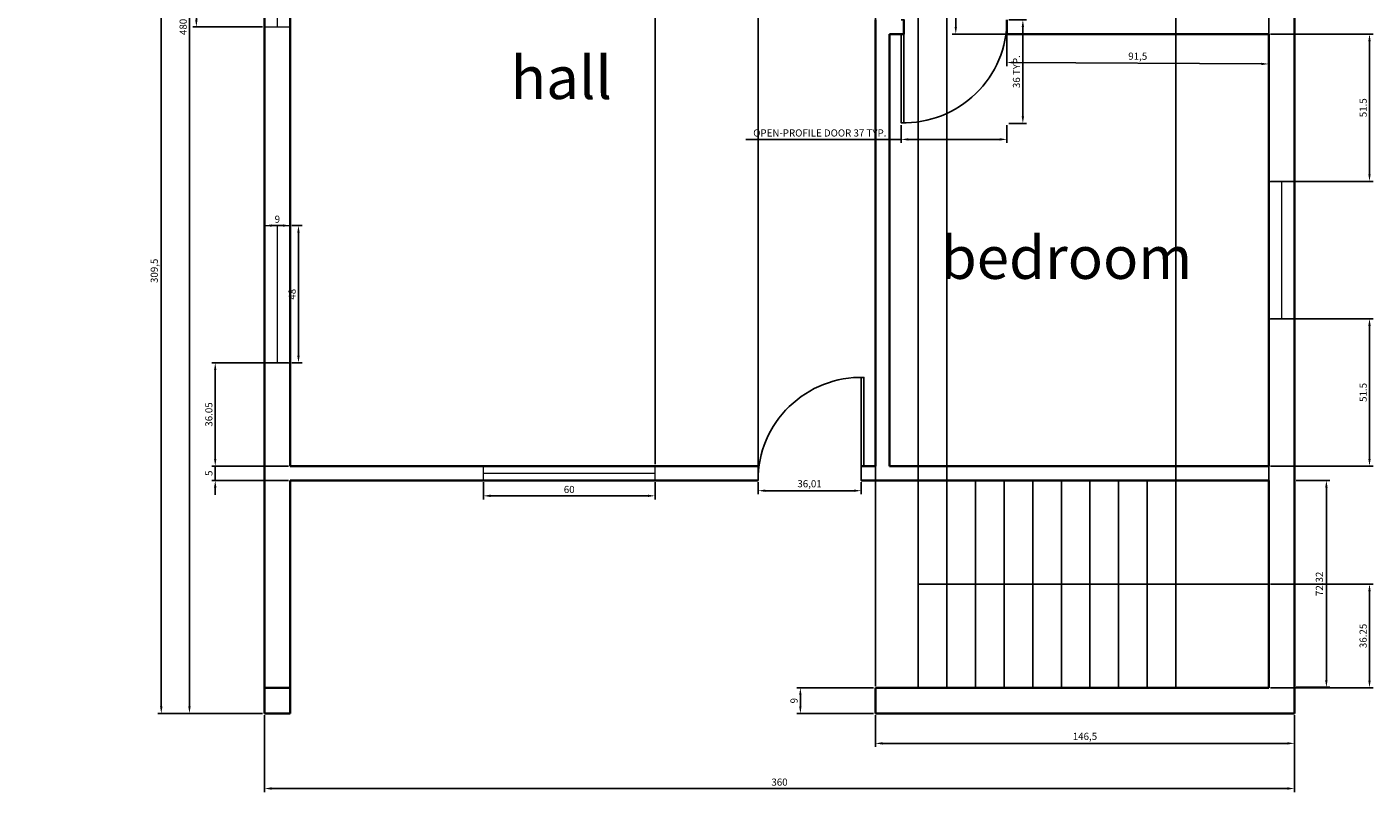
# Model space of a CAD drawing. Units: inches. Extents: x 64 to 791, y 453 to 990.
# Tile 1 of 3: x 314 to 784, y 453 to 721. Entities that reach past the tile are written whole.
import ezdxf

# ---------------------------------------------------------------- set-up
doc = ezdxf.new("R2010")
doc.units = ezdxf.units.IN
for name, color, linetype, lineweight in [('A-ANNO-DIMS', 2, 'Continuous', 18), ('A-AREA-IDEN', 7, 'Continuous', 25), ('A-DOOR', 3, 'Continuous', 25), ('A-FLOR-STRS', 8, 'Continuous', 25), ('A-GLAZ', 4, 'Continuous', 18), ('A-WALL', 7, 'Continuous', 35)]:
    doc.layers.add(name, color=color, linetype=linetype, lineweight=lineweight)
doc.styles.get("Standard").update_dxf_attribs({"font": 'arial.ttf'})
doc.dimstyles.new('ISO-25', dxfattribs={"dimtxt": 2.5, "dimasz": 2.5, "dimexe": 1.25, "dimexo": 0.625, "dimtad": 1, "dimtxsty": 'Standard', "dimcen": 2.5, "dimadec": 0, "dimazin": 0, "dimtfac": 1, "dimtmove": 0, "dimatfit": 3, "dimfxl": 1, "dimarcsym": 0})

# ---------------------------------------------------------------- blocks, each defined once
blk = doc.blocks.new('*D9')
at = {"layer": 'A-ANNO-DIMS', "color": 0, "lineweight": -2, "transparency": 16777216}
for p, q in [((757.56, 562.18), (769.32, 562.18)), ((768.07, 559.68), (768.07, 492.37)), ((757.56, 489.87), (769.32, 489.87))]:
    blk.add_line(p, q, dxfattribs=at)
at = {"layer": 'A-ANNO-DIMS', "color": 0, "transparency": 16777216}
for points in [[(767.65, 559.68), (768.48, 559.68), (768.07, 562.18)], [(767.65, 492.37), (768.48, 492.37), (768.07, 489.87)]]:
    blk.add_solid(points, dxfattribs=at)
at = {"layer": 'Defpoints', "color": 0, "transparency": 16777216}
for p in [(756.94, 562.18), (756.94, 489.87), (768.07, 489.87)]:
    blk.add_point(p, dxfattribs=at)
at = {"layer": 'A-ANNO-DIMS', "color": 0, "transparency": 16777216, "insert": (765.94, 526.02), "char_height": 2.5, "attachment_point": 5, "rotation": 90}
blk.add_mtext('72,32', dxfattribs=at)
blk = doc.blocks.new('*D10')
at = {"layer": 'A-ANNO-DIMS', "color": 0, "lineweight": -2, "transparency": 16777216}
for p, q in [((610.44, 480.06), (610.44, 469.01)), ((756.94, 480.06), (756.94, 469.01)), ((612.94, 470.26), (754.44, 470.26))]:
    blk.add_line(p, q, dxfattribs=at)
at = {"layer": 'A-ANNO-DIMS', "color": 0, "transparency": 16777216}
for points in [[(612.94, 470.67), (612.94, 469.84), (610.44, 470.26)], [(754.44, 470.67), (754.44, 469.84), (756.94, 470.26)]]:
    blk.add_solid(points, dxfattribs=at)
at = {"layer": 'Defpoints', "color": 0, "transparency": 16777216}
for p in [(610.44, 480.68), (756.94, 480.68), (756.94, 470.26)]:
    blk.add_point(p, dxfattribs=at)
at = {"layer": 'A-ANNO-DIMS', "color": 0, "transparency": 16777216, "insert": (683.69, 472.39), "char_height": 2.5, "attachment_point": 5}
blk.add_mtext('146,5', dxfattribs=at)
blk = doc.blocks.new('*D14')
at = {"layer": 'A-ANNO-DIMS', "color": 0, "lineweight": -2, "transparency": 16777216}
for p, q in [((396.31, 768.68), (371.89, 768.68)), ((373.14, 766.18), (373.14, 723.18)), ((396.31, 720.68), (371.89, 720.68))]:
    blk.add_line(p, q, dxfattribs=at)
at = {"layer": 'A-ANNO-DIMS', "color": 0, "transparency": 16777216}
for points in [[(372.72, 766.18), (373.55, 766.18), (373.14, 768.68)], [(372.72, 723.18), (373.55, 723.18), (373.14, 720.68)]]:
    blk.add_solid(points, dxfattribs=at)
at = {"layer": 'Defpoints', "color": 0, "transparency": 16777216}
for p in [(396.94, 768.68), (373.14, 720.68), (396.94, 720.68)]:
    blk.add_point(p, dxfattribs=at)
at = {"layer": 'A-ANNO-DIMS', "color": 0, "transparency": 16777216, "insert": (371.24, 744.68), "char_height": 2.5, "attachment_point": 5, "rotation": 90}
blk.add_mtext('48', dxfattribs=at)
blk = doc.blocks.new('*D15')
at = {"layer": 'A-ANNO-DIMS', "color": 0, "lineweight": -2, "transparency": 16777216}
for p, q in [((396.94, 603.86), (396.94, 652.49)), ((399.44, 651.24), (403.44, 651.24)), ((405.94, 603.86), (405.94, 652.49))]:
    blk.add_line(p, q, dxfattribs=at)
at = {"layer": 'A-ANNO-DIMS', "color": 0, "transparency": 16777216}
for points in [[(399.44, 651.65), (399.44, 650.82), (396.94, 651.24)], [(403.44, 651.65), (403.44, 650.82), (405.94, 651.24)]]:
    blk.add_solid(points, dxfattribs=at)
at = {"layer": 'Defpoints', "color": 0, "transparency": 16777216}
for p in [(405.94, 651.24), (396.94, 603.24), (405.94, 603.24)]:
    blk.add_point(p, dxfattribs=at)
at = {"layer": 'A-ANNO-DIMS', "color": 0, "transparency": 16777216, "insert": (401.44, 653.14), "char_height": 2.5, "attachment_point": 5}
blk.add_mtext('9', dxfattribs=at)
blk = doc.blocks.new('*D16')
at = {"layer": 'A-ANNO-DIMS', "color": 0, "lineweight": -2, "transparency": 16777216}
for p, q in [((406.56, 651.24), (410.08, 651.24)), ((408.83, 605.74), (408.83, 648.74)), ((406.56, 603.24), (410.08, 603.24))]:
    blk.add_line(p, q, dxfattribs=at)
at = {"layer": 'A-ANNO-DIMS', "color": 0, "transparency": 16777216}
for points in [[(408.41, 648.74), (409.24, 648.74), (408.83, 651.24)], [(408.41, 605.74), (409.24, 605.74), (408.83, 603.24)]]:
    blk.add_solid(points, dxfattribs=at)
at = {"layer": 'Defpoints', "color": 0, "transparency": 16777216}
for p in [(405.94, 651.24), (408.83, 651.24), (405.94, 603.24)]:
    blk.add_point(p, dxfattribs=at)
at = {"layer": 'A-ANNO-DIMS', "color": 0, "transparency": 16777216, "insert": (406.93, 627.24), "char_height": 2.5, "attachment_point": 5, "rotation": 90}
blk.add_mtext('48', dxfattribs=at)
blk = doc.blocks.new('*D17')
at = {"layer": 'A-ANNO-DIMS', "color": 0, "lineweight": -2, "transparency": 16777216}
for p, q in [((473.44, 561.56), (473.44, 555.53)), ((533.44, 561.56), (533.44, 555.53)), ((475.94, 556.78), (530.94, 556.78))]:
    blk.add_line(p, q, dxfattribs=at)
at = {"layer": 'A-ANNO-DIMS', "color": 0, "transparency": 16777216}
for points in [[(475.94, 557.2), (475.94, 556.37), (473.44, 556.78)], [(530.94, 557.2), (530.94, 556.37), (533.44, 556.78)]]:
    blk.add_solid(points, dxfattribs=at)
at = {"layer": 'Defpoints', "color": 0, "transparency": 16777216}
for p in [(473.44, 562.18), (533.44, 562.18), (533.44, 556.78)]:
    blk.add_point(p, dxfattribs=at)
at = {"layer": 'A-ANNO-DIMS', "color": 0, "transparency": 16777216, "insert": (503.44, 558.68), "char_height": 2.5, "attachment_point": 5}
blk.add_mtext('60', dxfattribs=at)
blk = doc.blocks.new('*D18')
at = {"layer": 'A-ANNO-DIMS', "color": 0, "lineweight": -2, "transparency": 16777216}
for p, q in [((569.44, 561.56), (569.44, 557.33)), ((605.45, 561.56), (605.45, 557.33)), ((571.94, 558.58), (602.95, 558.58))]:
    blk.add_line(p, q, dxfattribs=at)
at = {"layer": 'A-ANNO-DIMS', "color": 0, "transparency": 16777216}
for points in [[(571.94, 558.99), (571.94, 558.16), (569.44, 558.58)], [(602.95, 558.99), (602.95, 558.16), (605.45, 558.58)]]:
    blk.add_solid(points, dxfattribs=at)
at = {"layer": 'Defpoints', "color": 0, "transparency": 16777216}
for p in [(569.44, 562.18), (605.45, 562.18), (605.45, 558.58)]:
    blk.add_point(p, dxfattribs=at)
at = {"layer": 'A-ANNO-DIMS', "color": 0, "transparency": 16777216, "insert": (587.44, 560.7), "char_height": 2.5, "attachment_point": 5}
blk.add_mtext('36,01', dxfattribs=at)
blk = doc.blocks.new('*D22')
at = {"layer": 'A-ANNO-DIMS', "color": 0, "lineweight": -2, "transparency": 16777216}
for p, q in [((396.31, 790.18), (359.63, 790.18)), ((360.88, 483.18), (360.88, 787.68)), ((396.31, 480.68), (359.63, 480.68))]:
    blk.add_line(p, q, dxfattribs=at)
at = {"layer": 'A-ANNO-DIMS', "color": 0, "transparency": 16777216}
for points in [[(360.46, 787.68), (361.29, 787.68), (360.88, 790.18)], [(360.46, 483.18), (361.29, 483.18), (360.88, 480.68)]]:
    blk.add_solid(points, dxfattribs=at)
at = {"layer": 'Defpoints', "color": 0, "transparency": 16777216}
for p in [(360.88, 790.18), (396.94, 790.18), (396.94, 480.68)]:
    blk.add_point(p, dxfattribs=at)
at = {"layer": 'A-ANNO-DIMS', "color": 0, "transparency": 16777216, "insert": (358.75, 635.43), "char_height": 2.5, "attachment_point": 5, "rotation": 90}
blk.add_mtext('309,5', dxfattribs=at)
blk = doc.blocks.new('*D23')
at = {"layer": 'A-ANNO-DIMS', "color": 0, "lineweight": -2, "transparency": 16777216}
for p, q in [((655.81, 807.18), (637.3, 807.18)), ((638.55, 720.68), (638.55, 804.68)), ((655.81, 718.18), (637.3, 718.18))]:
    blk.add_line(p, q, dxfattribs=at)
at = {"layer": 'A-ANNO-DIMS', "color": 0, "transparency": 16777216}
for points in [[(638.13, 804.68), (638.96, 804.68), (638.55, 807.18)], [(638.13, 720.68), (638.96, 720.68), (638.55, 718.18)]]:
    blk.add_solid(points, dxfattribs=at)
at = {"layer": 'Defpoints', "color": 0, "transparency": 16777216}
for p in [(638.55, 807.18), (656.44, 807.18), (656.44, 718.18)]:
    blk.add_point(p, dxfattribs=at)
at = {"layer": 'A-ANNO-DIMS', "color": 0, "transparency": 16777216, "insert": (636.64, 762.68), "char_height": 2.5, "attachment_point": 5, "rotation": 90}
blk.add_mtext('89', dxfattribs=at)
blk = doc.blocks.new('*D24')
at = {"layer": 'A-ANNO-DIMS', "color": 0, "lineweight": -2, "transparency": 16777216}
for p, q in [((656.43, 718.08), (656.37, 707)), ((747.93, 717.56), (747.87, 706.48)), ((745.38, 707.74), (658.88, 708.24))]:
    blk.add_line(p, q, dxfattribs=at)
at = {"layer": 'A-ANNO-DIMS', "color": 0, "transparency": 16777216}
for points in [[(658.88, 708.65), (658.87, 707.82), (656.38, 708.25)], [(745.38, 708.16), (745.37, 707.32), (747.88, 707.73)]]:
    blk.add_solid(points, dxfattribs=at)
at = {"layer": 'Defpoints', "color": 0, "transparency": 16777216}
for p in [(656.44, 718.71), (747.94, 718.18), (656.38, 708.25)]:
    blk.add_point(p, dxfattribs=at)
at = {"layer": 'A-ANNO-DIMS', "color": 0, "transparency": 16777216, "insert": (702.14, 710.12), "char_height": 2.5, "attachment_point": 5, "rotation": 359.6705}
blk.add_mtext('91,5', dxfattribs=at)
blk = doc.blocks.new('WIN-48IN')
for p, q in [((0, 48), (9, 48)), ((4.5, 48), (4.5, 0)), ((0, 0), (9, 0))]:
    blk.add_line(p, q)
blk = doc.blocks.new('DOOR-SWING-36IN-OPEN-PROFILE')
for p, q in [((0, 0), (0, 5)), ((36, 0), (36, 5))]:
    blk.add_line(p, q)
blk.add_lwpolyline([(37, 5), (37, 36), (36, 36), (36, 0), (37, 0)])
blk.add_arc((36.01, 0), 36.01, 88.4304, 180)
blk = doc.blocks.new('*D30')
at = {"layer": 'A-ANNO-DIMS', "color": 0, "lineweight": -2, "transparency": 16777216}
for p, q in [((619.44, 686.29), (619.44, 680.12)), ((656.44, 686.29), (656.44, 680.12)), ((619.44, 681.37), (565.12, 681.37)), ((653.94, 681.37), (621.94, 681.37))]:
    blk.add_line(p, q, dxfattribs=at)
at = {"layer": 'A-ANNO-DIMS', "color": 0, "transparency": 16777216}
for points in [[(621.94, 681.78), (621.94, 680.95), (619.44, 681.37)], [(653.94, 681.78), (653.94, 680.95), (656.44, 681.37)]]:
    blk.add_solid(points, dxfattribs=at)
at = {"layer": 'Defpoints', "color": 0, "transparency": 16777216}
for p in [(619.44, 686.92), (656.44, 686.92), (619.44, 681.37)]:
    blk.add_point(p, dxfattribs=at)
at = {"layer": 'A-ANNO-DIMS', "color": 0, "transparency": 16777216, "insert": (591.03, 683.29), "char_height": 2.5, "attachment_point": 5}
blk.add_mtext('OPEN-PROFILE DOOR 37 TYP.', dxfattribs=at)
blk = doc.blocks.new('*D31')
at = {"layer": 'A-ANNO-DIMS', "color": 0, "lineweight": -2, "transparency": 16777216}
for p, q in [((657.06, 723.18), (663.24, 723.18)), ((661.99, 720.68), (661.99, 689.42)), ((657.06, 686.92), (663.24, 686.92))]:
    blk.add_line(p, q, dxfattribs=at)
at = {"layer": 'A-ANNO-DIMS', "color": 0, "transparency": 16777216}
for points in [[(661.57, 720.68), (662.4, 720.68), (661.99, 723.18)], [(661.57, 689.42), (662.4, 689.42), (661.99, 686.92)]]:
    blk.add_solid(points, dxfattribs=at)
at = {"layer": 'Defpoints', "color": 0, "transparency": 16777216}
for p in [(656.44, 723.18), (656.44, 686.92), (661.99, 686.92)]:
    blk.add_point(p, dxfattribs=at)
at = {"layer": 'A-ANNO-DIMS', "color": 0, "transparency": 16777216, "insert": (660.08, 705.05), "char_height": 2.5, "attachment_point": 5, "rotation": 90}
blk.add_mtext('36 TYP.', dxfattribs=at)
blk = doc.blocks.new('*D32')
at = {"layer": 'A-ANNO-DIMS', "color": 0, "lineweight": -2, "transparency": 16777216}
for p, q in [((396.94, 480.06), (396.94, 453.23)), ((756.94, 480.06), (756.94, 453.23)), ((399.44, 454.48), (754.44, 454.48))]:
    blk.add_line(p, q, dxfattribs=at)
at = {"layer": 'A-ANNO-DIMS', "color": 0, "transparency": 16777216}
for points in [[(399.44, 454.9), (399.44, 454.07), (396.94, 454.48)], [(754.44, 454.9), (754.44, 454.07), (756.94, 454.48)]]:
    blk.add_solid(points, dxfattribs=at)
at = {"layer": 'Defpoints', "color": 0, "transparency": 16777216}
for p in [(396.94, 480.68), (756.94, 480.68), (756.94, 454.48)]:
    blk.add_point(p, dxfattribs=at)
at = {"layer": 'A-ANNO-DIMS', "color": 0, "transparency": 16777216, "insert": (576.94, 456.39), "char_height": 2.5, "attachment_point": 5}
blk.add_mtext('360', dxfattribs=at)
blk = doc.blocks.new('*D33')
at = {"layer": 'A-ANNO-DIMS', "color": 0, "lineweight": -2, "transparency": 16777216}
for p, q in [((396.31, 960.68), (369.49, 960.68)), ((370.74, 483.18), (370.74, 958.18)), ((396.31, 480.68), (369.49, 480.68))]:
    blk.add_line(p, q, dxfattribs=at)
at = {"layer": 'A-ANNO-DIMS', "color": 0, "transparency": 16777216}
for points in [[(370.32, 958.18), (371.15, 958.18), (370.74, 960.68)], [(370.32, 483.18), (371.15, 483.18), (370.74, 480.68)]]:
    blk.add_solid(points, dxfattribs=at)
at = {"layer": 'Defpoints', "color": 0, "transparency": 16777216}
for p in [(370.74, 960.68), (396.94, 960.68), (396.94, 480.68)]:
    blk.add_point(p, dxfattribs=at)
at = {"layer": 'A-ANNO-DIMS', "color": 0, "transparency": 16777216, "insert": (368.84, 720.68), "char_height": 2.5, "attachment_point": 5, "rotation": 90}
blk.add_mtext('480', dxfattribs=at)
blk = doc.blocks.new('*D36')
at = {"layer": 'A-ANNO-DIMS', "color": 0, "lineweight": -2, "transparency": 16777216}
for p, q in [((748.56, 718.18), (784.39, 718.18)), ((783.14, 669.18), (783.14, 715.68)), ((748.56, 666.68), (784.39, 666.68))]:
    blk.add_line(p, q, dxfattribs=at)
at = {"layer": 'A-ANNO-DIMS', "color": 0, "transparency": 16777216}
for points in [[(782.72, 715.68), (783.55, 715.68), (783.14, 718.18)], [(782.72, 669.18), (783.55, 669.18), (783.14, 666.68)]]:
    blk.add_solid(points, dxfattribs=at)
at = {"layer": 'Defpoints', "color": 0, "transparency": 16777216}
for p in [(747.94, 718.18), (783.14, 718.18), (747.94, 666.68)]:
    blk.add_point(p, dxfattribs=at)
at = {"layer": 'A-ANNO-DIMS', "color": 0, "transparency": 16777216, "insert": (781.24, 692.43), "char_height": 2.5, "attachment_point": 5, "rotation": 90}
blk.add_mtext('51.5', dxfattribs=at)
blk = doc.blocks.new('*D39')
at = {"layer": 'A-ANNO-DIMS', "color": 0, "lineweight": -2, "transparency": 16777216}
for p, q in [((405.31, 603.24), (378.49, 603.24)), ((379.74, 569.68), (379.74, 600.74)), ((405.31, 567.18), (378.49, 567.18))]:
    blk.add_line(p, q, dxfattribs=at)
at = {"layer": 'A-ANNO-DIMS', "color": 0, "transparency": 16777216}
for points in [[(379.32, 600.74), (380.15, 600.74), (379.74, 603.24)], [(379.32, 569.68), (380.15, 569.68), (379.74, 567.18)]]:
    blk.add_solid(points, dxfattribs=at)
at = {"layer": 'Defpoints', "color": 0, "transparency": 16777216}
for p in [(379.74, 603.24), (405.94, 603.24), (405.94, 567.18)]:
    blk.add_point(p, dxfattribs=at)
at = {"layer": 'A-ANNO-DIMS', "color": 0, "transparency": 16777216, "insert": (377.83, 585.21), "char_height": 2.5, "attachment_point": 5, "rotation": 90}
blk.add_mtext('36.05', dxfattribs=at)
blk = doc.blocks.new('*D40')
at = {"layer": 'A-ANNO-DIMS', "color": 0, "lineweight": -2, "transparency": 16777216}
for p, q in [((748.56, 618.68), (784.39, 618.68)), ((783.14, 569.68), (783.14, 616.18)), ((748.56, 567.18), (784.39, 567.18))]:
    blk.add_line(p, q, dxfattribs=at)
at = {"layer": 'A-ANNO-DIMS', "color": 0, "transparency": 16777216}
for points in [[(782.72, 616.18), (783.55, 616.18), (783.14, 618.68)], [(782.72, 569.68), (783.55, 569.68), (783.14, 567.18)]]:
    blk.add_solid(points, dxfattribs=at)
at = {"layer": 'Defpoints', "color": 0, "transparency": 16777216}
for p in [(747.94, 618.68), (783.14, 618.68), (747.94, 567.18)]:
    blk.add_point(p, dxfattribs=at)
at = {"layer": 'A-ANNO-DIMS', "color": 0, "transparency": 16777216, "insert": (781.24, 592.93), "char_height": 2.5, "attachment_point": 5, "rotation": 90}
blk.add_mtext('51.5', dxfattribs=at)
blk = doc.blocks.new('*D43')
at = {"layer": 'A-ANNO-DIMS', "color": 0, "lineweight": -2, "transparency": 16777216}
for p, q in [((569.44, 562.81), (569.44, 988.13)), ((610.44, 567.81), (610.44, 988.13)), ((571.94, 986.88), (607.94, 986.88))]:
    blk.add_line(p, q, dxfattribs=at)
at = {"layer": 'A-ANNO-DIMS', "color": 0, "transparency": 16777216}
for points in [[(571.94, 987.3), (571.94, 986.47), (569.44, 986.88)], [(607.94, 987.3), (607.94, 986.47), (610.44, 986.88)]]:
    blk.add_solid(points, dxfattribs=at)
at = {"layer": 'Defpoints', "color": 0, "transparency": 16777216}
for p in [(610.44, 986.88), (610.44, 567.18), (569.44, 562.18)]:
    blk.add_point(p, dxfattribs=at)
at = {"layer": 'A-ANNO-DIMS', "color": 0, "transparency": 16777216, "insert": (589.94, 988.76), "char_height": 2.5, "attachment_point": 5}
blk.add_mtext('41', dxfattribs=at)
blk = doc.blocks.new('*D44')
at = {"layer": 'A-ANNO-DIMS', "color": 0, "lineweight": -2, "transparency": 16777216}
for p, q in [((533.44, 567.81), (533.44, 988.13)), ((569.44, 562.81), (569.44, 988.13)), ((535.94, 986.88), (566.94, 986.88))]:
    blk.add_line(p, q, dxfattribs=at)
at = {"layer": 'A-ANNO-DIMS', "color": 0, "transparency": 16777216}
for points in [[(535.94, 987.3), (535.94, 986.47), (533.44, 986.88)], [(566.94, 987.3), (566.94, 986.47), (569.44, 986.88)]]:
    blk.add_solid(points, dxfattribs=at)
at = {"layer": 'Defpoints', "color": 0, "transparency": 16777216}
for p in [(569.44, 986.88), (533.44, 567.18), (569.44, 562.18)]:
    blk.add_point(p, dxfattribs=at)
at = {"layer": 'A-ANNO-DIMS', "color": 0, "transparency": 16777216, "insert": (551.44, 988.79), "char_height": 2.5, "attachment_point": 5}
blk.add_mtext('36', dxfattribs=at)
blk = doc.blocks.new('*D45')
at = {"layer": 'A-ANNO-DIMS', "color": 0, "lineweight": -2, "transparency": 16777216}
for p, q in [((625.44, 490.31), (625.44, 988.13)), ((635.44, 490.31), (635.44, 988.13)), ((627.94, 986.88), (632.94, 986.88))]:
    blk.add_line(p, q, dxfattribs=at)
at = {"layer": 'A-ANNO-DIMS', "color": 0, "transparency": 16777216}
for points in [[(627.94, 987.3), (627.94, 986.47), (625.44, 986.88)], [(632.94, 987.3), (632.94, 986.47), (635.44, 986.88)]]:
    blk.add_solid(points, dxfattribs=at)
at = {"layer": 'Defpoints', "color": 0, "transparency": 16777216}
for p in [(635.44, 986.88), (625.44, 489.68), (635.44, 489.68)]:
    blk.add_point(p, dxfattribs=at)
at = {"layer": 'A-ANNO-DIMS', "color": 0, "transparency": 16777216, "insert": (630.44, 988.78), "char_height": 2.5, "attachment_point": 5}
blk.add_mtext('10', dxfattribs=at)
blk = doc.blocks.new('*D46')
at = {"layer": 'A-ANNO-DIMS', "color": 0, "lineweight": -2, "transparency": 16777216}
for p, q in [((610.44, 490.31), (610.44, 988.13)), ((625.44, 490.31), (625.44, 988.13)), ((612.94, 986.88), (622.94, 986.88))]:
    blk.add_line(p, q, dxfattribs=at)
at = {"layer": 'A-ANNO-DIMS', "color": 0, "transparency": 16777216}
for points in [[(612.94, 987.3), (612.94, 986.47), (610.44, 986.88)], [(622.94, 987.3), (622.94, 986.47), (625.44, 986.88)]]:
    blk.add_solid(points, dxfattribs=at)
at = {"layer": 'Defpoints', "color": 0, "transparency": 16777216}
for p in [(625.44, 986.88), (610.44, 489.68), (625.44, 489.68)]:
    blk.add_point(p, dxfattribs=at)
at = {"layer": 'A-ANNO-DIMS', "color": 0, "transparency": 16777216, "insert": (617.94, 988.78), "char_height": 2.5, "attachment_point": 5}
blk.add_mtext('15', dxfattribs=at)
blk = doc.blocks.new('*D47')
at = {"layer": 'A-ANNO-DIMS', "color": 0, "lineweight": -2, "transparency": 16777216}
for p, q in [((715.44, 490.31), (715.44, 988.13)), ((747.94, 490.31), (747.94, 988.13)), ((717.94, 986.88), (745.44, 986.88))]:
    blk.add_line(p, q, dxfattribs=at)
at = {"layer": 'A-ANNO-DIMS', "color": 0, "transparency": 16777216}
for points in [[(717.94, 987.3), (717.94, 986.47), (715.44, 986.88)], [(745.44, 987.3), (745.44, 986.47), (747.94, 986.88)]]:
    blk.add_solid(points, dxfattribs=at)
at = {"layer": 'Defpoints', "color": 0, "transparency": 16777216}
for p in [(747.94, 986.88), (715.44, 489.68), (747.94, 489.68)]:
    blk.add_point(p, dxfattribs=at)
at = {"layer": 'A-ANNO-DIMS', "color": 0, "transparency": 16777216, "insert": (731.69, 988.79), "char_height": 2.5, "attachment_point": 5}
blk.add_mtext('32.5', dxfattribs=at)
blk = doc.blocks.new('*D48')
at = {"layer": 'A-ANNO-DIMS', "color": 0, "lineweight": -2, "transparency": 16777216}
for p, q in [((748.56, 525.93), (784.39, 525.93)), ((783.14, 492.18), (783.14, 523.43)), ((748.56, 489.68), (784.39, 489.68))]:
    blk.add_line(p, q, dxfattribs=at)
at = {"layer": 'A-ANNO-DIMS', "color": 0, "transparency": 16777216}
for points in [[(782.72, 523.43), (783.55, 523.43), (783.14, 525.93)], [(782.72, 492.18), (783.55, 492.18), (783.14, 489.68)]]:
    blk.add_solid(points, dxfattribs=at)
at = {"layer": 'Defpoints', "color": 0, "transparency": 16777216}
for p in [(747.94, 525.93), (783.14, 525.93), (747.94, 489.68)]:
    blk.add_point(p, dxfattribs=at)
at = {"layer": 'A-ANNO-DIMS', "color": 0, "transparency": 16777216, "insert": (781.23, 507.81), "char_height": 2.5, "attachment_point": 5, "rotation": 90}
blk.add_mtext('36.25', dxfattribs=at)
blk = doc.blocks.new('*D53')
at = {"layer": 'A-ANNO-DIMS', "color": 0, "lineweight": -2, "transparency": 16777216}
for p, q in [((609.81, 489.68), (582.99, 489.68)), ((584.24, 483.18), (584.24, 487.18)), ((609.81, 480.68), (582.99, 480.68))]:
    blk.add_line(p, q, dxfattribs=at)
at = {"layer": 'A-ANNO-DIMS', "color": 0, "transparency": 16777216}
for points in [[(583.82, 487.18), (584.65, 487.18), (584.24, 489.68)], [(583.82, 483.18), (584.65, 483.18), (584.24, 480.68)]]:
    blk.add_solid(points, dxfattribs=at)
at = {"layer": 'Defpoints', "color": 0, "transparency": 16777216}
for p in [(584.24, 489.68), (610.44, 489.68), (610.44, 480.68)]:
    blk.add_point(p, dxfattribs=at)
at = {"layer": 'A-ANNO-DIMS', "color": 0, "transparency": 16777216, "insert": (582.34, 485.18), "char_height": 2.5, "attachment_point": 5, "rotation": 90}
blk.add_mtext('9', dxfattribs=at)
blk = doc.blocks.new('*D54')
at = {"layer": 'A-ANNO-DIMS', "color": 0, "lineweight": -2, "transparency": 16777216}
for p, q in [((379.74, 569.68), (379.74, 572.18)), ((405.31, 567.18), (378.49, 567.18)), ((379.74, 562.18), (379.74, 567.18)), ((405.31, 562.18), (378.49, 562.18)), ((379.74, 559.68), (379.74, 557.18))]:
    blk.add_line(p, q, dxfattribs=at)
at = {"layer": 'A-ANNO-DIMS', "color": 0, "transparency": 16777216}
for points in [[(379.32, 569.68), (380.15, 569.68), (379.74, 567.18)], [(379.32, 559.68), (380.15, 559.68), (379.74, 562.18)]]:
    blk.add_solid(points, dxfattribs=at)
at = {"layer": 'Defpoints', "color": 0, "transparency": 16777216}
for p in [(379.74, 567.18), (405.94, 567.18), (405.94, 562.18)]:
    blk.add_point(p, dxfattribs=at)
at = {"layer": 'A-ANNO-DIMS', "color": 0, "transparency": 16777216, "insert": (377.84, 564.68), "char_height": 2.5, "attachment_point": 5, "rotation": 90}
blk.add_mtext('5', dxfattribs=at)

msp = doc.modelspace()

# ---------------------------------------------------------------- linework, layer by layer
at = {"layer": 'A-DOOR'}
msp.add_arc((349.9365, 562.1832), 36.0135, 359.9999999999988, 0, dxfattribs=at)
at = {"layer": 'A-FLOR-STRS'}
for p, q in [((625.437, 489.6832), (625.437, 562.1832)), ((635.437, 489.6832), (635.437, 562.1832)), ((645.437, 489.6832), (645.437, 562.1832)), ((655.437, 489.6832), (655.437, 562.1832)), ((665.437, 489.6832), (665.437, 562.1832)), ((675.437, 489.6832), (675.437, 562.1832)), ((685.437, 489.6832), (685.437, 562.1832)), ((695.437, 489.6832), (695.437, 562.1832)), ((705.437, 489.6832), (705.437, 562.1832)), ((715.437, 489.6832), (715.437, 562.1832)), ((625.437, 525.9332), (747.937, 525.9332))]:
    msp.add_line(p, q, dxfattribs=at)
at = {"layer": 'A-GLAZ'}
for p, q in [((473.437, 562.1832), (473.437, 567.1832)), ((473.437, 564.6832), (533.437, 564.6832)), ((503.437, 564.6832), (503.437, 564.6832)), ((533.437, 562.1832), (533.437, 567.1832))]:
    msp.add_line(p, q, dxfattribs=at)
at = {"layer": 'A-WALL'}
for p, q in [((396.937, 960.6832), (396.937, 480.6832)), ((756.937, 480.6832), (756.937, 960.6832)), ((756.937, 804.6832), (756.937, 720.6832)), ((405.937, 790.1832), (405.937, 567.1832)), ((610.437, 723.1832), (610.437, 720.6832)), ((610.437, 567.1832), (610.437, 720.6832)), ((620.437, 718.1832), (620.437, 723.1832)), ((656.437, 718.1832), (656.437, 723.1832)), ((615.437, 718.1832), (620.437, 718.1832)), ((615.437, 567.1832), (615.437, 718.1832)), ((656.437, 718.1832), (747.937, 718.1832)), ((747.937, 718.1832), (747.937, 567.1832)), ((747.937, 567.1832), (747.937, 718.1832)), ((747.937, 567.1832), (747.937, 718.1832)), ((405.937, 567.1832), (569.437, 567.1832)), ((605.437, 567.1832), (610.437, 567.1832)), ((615.437, 567.1832), (747.937, 567.1832)), ((405.937, 562.1832), (569.437, 562.1832)), ((405.937, 562.1832), (405.937, 480.6832)), ((605.437, 562.1832), (610.437, 562.1832)), ((615.437, 562.1832), (610.437, 562.1832)), ((615.437, 562.1832), (747.937, 562.1832)), ((747.937, 489.6832), (747.937, 562.1832)), ((396.937, 489.6832), (405.937, 489.6832)), ((610.437, 480.6832), (610.437, 489.6832)), ((610.437, 489.6832), (747.937, 489.6832)), ((396.937, 480.6832), (405.937, 480.6832)), ((610.437, 480.6832), (756.937, 480.6832))]:
    msp.add_line(p, q, dxfattribs=at)

# ---------------------------------------------------------------- block references
at = {"layer": 'A-DOOR', "rotation": 180}
msp.add_blockref('DOOR-SWING-36IN-OPEN-PROFILE', (656.437, 723.1834), dxfattribs=at)
at = {"layer": 'A-DOOR'}
msp.add_blockref('DOOR-SWING-36IN-OPEN-PROFILE', (569.437, 562.183), dxfattribs=at)
at = {"layer": 'A-GLAZ'}
for p in [(396.937, 720.6828), (747.937, 618.6828), (396.937, 603.236)]:
    msp.add_blockref('WIN-48IN', p, dxfattribs=at)

# ---------------------------------------------------------------- texts
at = {"layer": 'A-AREA-IDEN'}
for s, p in [('hall', (483.0171, 695.4619)), ('bedroom', (633.2869, 632.6069))]:
    msp.add_text(s, height=14.92404, dxfattribs=at).set_placement(p)

# ---------------------------------------------------------------- dimensions: what is measured, and where the dimension line sits
at = {"layer": 'A-ANNO-DIMS'}
for base, p1, p2, override, picture, middle in [((569.437, 986.8832), (533.437, 567.1832), (569.437, 562.1832), {"dimdec": 0, "dimlfac": 1, "dimrnd": 0, "dimzin": 0, "dimdsep": 46, "dimlunit": 2}, '*D44', (551.437, 988.7855)), ((610.437, 986.8832), (569.437, 562.1832), (610.437, 567.1832), {"dimdec": 0, "dimlfac": 1, "dimrnd": 0, "dimzin": 0, "dimdsep": 46, "dimlunit": 2}, '*D43', (589.937, 988.7633)), ((625.437, 986.8832), (610.437, 489.6832), (625.437, 489.6832), {"dimdec": 0, "dimlfac": 1, "dimrnd": 0, "dimzin": 0, "dimdsep": 46, "dimlunit": 2}, '*D46', (617.937, 988.7846)), ((635.437, 986.8832), (625.437, 489.6832), (635.437, 489.6832), {"dimdec": 0, "dimlfac": 1, "dimrnd": 0, "dimzin": 0, "dimdsep": 46, "dimlunit": 2}, '*D45', (630.437, 988.7846)), ((747.937, 986.8832), (715.437, 489.6832), (747.937, 489.6832), {"dimdec": 1, "dimlfac": 1, "dimrnd": 0, "dimzin": 0, "dimdsep": 46, "dimlunit": 2}, '*D47', (731.687, 988.7855)), ((533.437, 556.7835), (473.437, 562.1832), (533.437, 562.1832), {"dimclrd": 0, "dimclre": 0, "dimclrt": 0}, '*D17', (503.437, 558.6849)), ((605.4505, 558.5767), (569.437, 562.1832), (605.4505, 562.1832), {"dimclrd": 0, "dimclre": 0, "dimclrt": 0}, '*D18', (587.4437, 560.704)), ((756.937, 454.4832), (396.937, 480.6832), (756.937, 480.6832), {"dimdec": 0, "dimlfac": 1, "dimrnd": 0, "dimzin": 0, "dimdsep": 46, "dimlunit": 2}, '*D32', (576.937, 456.3855)), ((756.937, 470.2577), (610.437, 480.6832), (756.937, 480.6832), {"dimclrd": 0, "dimclre": 0, "dimclrt": 0}, '*D10', (683.687, 472.3851))]:
    dim = msp.add_linear_dim(base=base, p1=p1, p2=p2, dimstyle='ISO-25', override=override, dxfattribs=at)
    dim.commit()
    dim.dimension.update_dxf_attribs({"geometry": picture, "text_midpoint": middle})
for base, p1, p2, override, picture, middle in [((370.737, 960.6832), (396.937, 480.6832), (396.937, 960.6832), {"dimdec": 0, "dimlfac": 1, "dimrnd": 0, "dimzin": 0, "dimdsep": 46, "dimlunit": 2}, '*D33', (368.8355, 720.6832)), ((638.5461, 807.1832), (656.437, 718.1832), (656.437, 807.1832), {"dimclrd": 0, "dimclre": 0, "dimclrt": 0}, '*D23', (636.6447, 762.6832)), ((360.8763, 790.1832), (396.937, 480.6832), (396.937, 790.1832), {"dimclrd": 0, "dimclre": 0, "dimclrt": 0}, '*D22', (358.749, 635.4332)), ((373.1367, 720.6832), (396.937, 768.6832), (396.937, 720.6832), {"dimclrd": 0, "dimclre": 0, "dimclrt": 0}, '*D14', (371.2352, 744.6832)), ((783.137, 718.1832), (747.937, 666.6832), (747.937, 718.1832), {"dimdec": 1, "dimlfac": 1, "dimrnd": 0, "dimzin": 0, "dimdsep": 46, "dimlunit": 2}, '*D36', (781.2355, 692.4332)), ((408.8283, 651.2364), (405.937, 603.2364), (405.937, 651.2364), {"dimclrd": 0, "dimclre": 0, "dimclrt": 0}, '*D16', (406.9268, 627.2364)), ((783.137, 618.6832), (747.937, 567.1832), (747.937, 618.6832), {"dimdec": 1, "dimlfac": 1, "dimrnd": 0, "dimzin": 0, "dimdsep": 46, "dimlunit": 2}, '*D40', (781.2355, 592.9332)), ((379.737, 603.2364), (405.937, 567.1832), (405.937, 603.2364), {"dimdec": 2, "dimlfac": 1, "dimrnd": 0, "dimzin": 0, "dimdsep": 46, "dimlunit": 2}, '*D39', (377.8347, 585.2098)), ((379.737, 567.1832), (405.937, 562.1832), (405.937, 567.1832), {"dimdec": 0, "dimlfac": 1, "dimrnd": 0, "dimzin": 0, "dimdsep": 46, "dimlunit": 2}, '*D54', (377.8407, 564.6832)), ((768.0681, 489.8653), (756.937, 562.1832), (756.937, 489.8653), {"dimclrd": 0, "dimclre": 0, "dimclrt": 0}, '*D9', (765.9407, 526.0242)), ((783.137, 525.9332), (747.937, 489.6832), (747.937, 525.9332), {"dimdec": 2, "dimlfac": 1, "dimrnd": 0, "dimzin": 0, "dimdsep": 46, "dimlunit": 2}, '*D48', (781.2347, 507.8082)), ((584.237, 489.6832), (610.437, 480.6832), (610.437, 489.6832), {"dimdec": 0, "dimlfac": 1, "dimrnd": 0, "dimzin": 0, "dimdsep": 46, "dimlunit": 2}, '*D53', (582.3355, 485.1832))]:
    dim = msp.add_linear_dim(base=base, p1=p1, p2=p2, angle=90, dimstyle='ISO-25', override=override, dxfattribs=at)
    dim.commit()
    dim.dimension.update_dxf_attribs({"geometry": picture, "text_midpoint": middle})
for base, p1, p2, angle, text, picture, middle in [((661.987, 686.9169), (656.437, 723.1832), (656.437, 686.9169), 270, '<> TYP.', '*D31', (660.0847, 705.0501)), ((619.437, 681.3669), (656.437, 686.9169), (619.437, 686.9169), 180, 'OPEN-PROFILE DOOR <> TYP.', '*D30', (591.028, 683.2862))]:
    dim = msp.add_linear_dim(base=base, p1=p1, p2=p2, angle=angle, text=text, dimstyle='ISO-25', override={"dimdec": 0, "dimlfac": 1, "dimrnd": 0, "dimzin": 0, "dimdsep": 46, "dimlunit": 2}, dxfattribs=at)
    dim.commit()
    dim.dimension.update_dxf_attribs({"geometry": picture, "text_midpoint": middle})
for p1, p2, distance, picture, middle in [((747.937, 718.1832), (656.437, 718.7094), 10.458, '*D24', (702.1391, 710.1159)), ((396.937, 603.2364), (405.937, 603.2364), 48, '*D15', (401.437, 653.1378))]:
    dim = msp.add_aligned_dim(p1=p1, p2=p2, distance=distance, dimstyle='ISO-25', override={"dimclrd": 0, "dimclre": 0, "dimclrt": 0}, dxfattribs=at)
    dim.commit()
    dim.dimension.update_dxf_attribs({"geometry": picture, "text_midpoint": middle})

doc.saveas('drawing.dxf')
